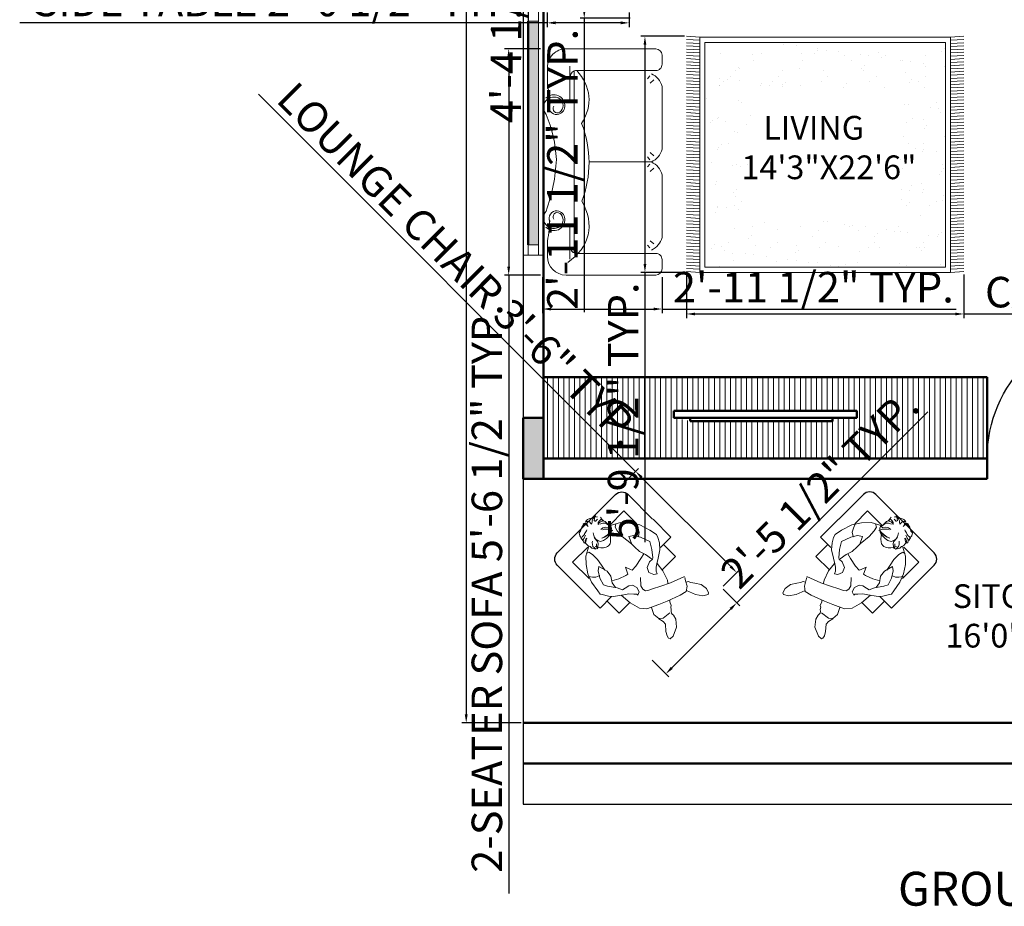
# Model space of a CAD drawing. Units: inches. Extents: x 3064 to 19385, y 846 to 15425.
# Tile 1 of 108: x 3072 to 3363, y 850 to 1112. Entities that reach past the tile are written whole.
import ezdxf

# ---------------------------------------------------------------- set-up
doc = ezdxf.new("R2010")
doc.units = ezdxf.units.IN
for name, color, linetype, lineweight in [('A-ANNO-DIMS', 2, 'Continuous', 18), ('A-ANNO-TEXT', 7, 'Continuous', 25), ('A-AREA-IDEN', 3, 'Continuous', 18), ('A-COLS', 1, 'Continuous', 35), ('A-DOOR', 3, 'Continuous', 25), ('A-FURN', 8, 'Continuous', 18), ('A-FURN-PATT', 252, 'Continuous', 13), ('A-GLAZ', 4, 'Continuous', 18), ('A-WALL', 7, 'Continuous', 50), ('C-PROP', 6, 'Continuous', 25)]:
    doc.layers.add(name, color=color, linetype=linetype, lineweight=lineweight)
doc.layers.add('NOITHAT', color=21, linetype='Continuous')
doc.styles.get("Standard").update_dxf_attribs({"font": 'arial.ttf'})
doc.dimstyles.new('ISO-25', dxfattribs={"dimtxt": 9, "dimasz": 2.5, "dimexe": 1.25, "dimexo": 0.625, "dimtad": 1, "dimdec": 1, "dimlunit": 3, "dimtxsty": 'Standard', "dimcen": 2.5, "dimadec": 0, "dimazin": 0, "dimtfac": 1, "dimtdec": 1, "dimtmove": 0, "dimatfit": 3, "dimfxl": 1, "dimarcsym": 0})

# ---------------------------------------------------------------- blocks, each defined once
blk = doc.blocks.new('*U2')
for p, q in [((0, 0), (0, -6)), ((40, 0), (40, -6))]:
    blk.add_line(p, q)
blk.add_lwpolyline([(0, 0), (0, 40), (1.75, 40), (1.75, 0)], close=True)
blk.add_arc((0, 0), 40, 0, 90)
blk = doc.blocks.new('carpet-9')
at = {"color": 0, "linetype": 'ByBlock'}
for p, q in [((-2.523, -0.142), (-2.531, 0)), ((-2.488, -0.142), (-2.497, 0)), ((-2.454, -0.142), (-2.462, 0)), ((-2.42, -0.142), (-2.428, 0)), ((-2.386, -0.142), (-2.394, 0)), ((-2.352, -0.142), (-2.36, 0)), ((-2.317, -0.142), (-2.326, 0)), ((-2.283, -0.142), (-2.291, 0)), ((-2.249, -0.142), (-2.257, 0)), ((-2.215, -0.142), (-2.223, 0)), ((-2.181, -0.142), (-2.189, 0)), ((-2.146, -0.142), (-2.155, 0)), ((-2.112, -0.142), (-2.12, 0)), ((-2.078, -0.142), (-2.086, 0)), ((-2.044, -0.142), (-2.052, 0)), ((-2.01, -0.142), (-2.018, 0)), ((-1.975, -0.142), (-1.984, 0)), ((-1.941, -0.142), (-1.949, 0)), ((-1.907, -0.142), (-1.915, 0)), ((-1.873, -0.142), (-1.881, 0)), ((-1.839, -0.142), (-1.847, 0)), ((-1.804, -0.142), (-1.813, 0)), ((-1.77, -0.142), (-1.778, 0)), ((-1.736, -0.142), (-1.744, 0)), ((-1.702, -0.142), (-1.71, 0)), ((-1.668, -0.142), (-1.676, 0)), ((-1.633, -0.142), (-1.642, 0)), ((-1.599, -0.142), (-1.607, 0)), ((-1.565, -0.142), (-1.573, 0)), ((-1.531, -0.142), (-1.539, 0)), ((-1.497, -0.142), (-1.505, 0)), ((-1.462, -0.142), (-1.471, 0)), ((-1.428, -0.142), (-1.436, 0)), ((-1.394, -0.142), (-1.402, 0)), ((-1.36, -0.142), (-1.368, 0)), ((-1.326, -0.142), (-1.334, 0)), ((-1.291, -0.142), (-1.3, 0)), ((-1.257, -0.142), (-1.265, 0)), ((-1.223, -0.142), (-1.231, 0)), ((-1.189, -0.142), (-1.197, 0)), ((-1.155, -0.142), (-1.163, 0)), ((-1.12, -0.142), (-1.129, 0)), ((-1.086, -0.142), (-1.094, 0)), ((-1.052, -0.142), (-1.06, 0)), ((-1.018, -0.142), (-1.026, 0)), ((-0.984, -0.142), (-0.992, 0)), ((-0.949, -0.142), (-0.958, 0)), ((-0.915, -0.142), (-0.923, 0)), ((-0.881, -0.142), (-0.889, 0)), ((-0.847, -0.142), (-0.855, 0)), ((-0.813, -0.142), (-0.821, 0)), ((-0.778, -0.142), (-0.787, 0)), ((-0.744, -0.142), (-0.752, 0)), ((-0.71, -0.142), (-0.718, 0)), ((-0.676, -0.142), (-0.684, 0)), ((-0.642, -0.142), (-0.65, 0)), ((-0.607, -0.142), (-0.616, 0)), ((-0.573, -0.142), (-0.581, 0)), ((-0.539, -0.142), (-0.547, 0)), ((-0.505, -0.142), (-0.513, 0)), ((-0.471, -0.142), (-0.479, 0)), ((-0.436, -0.142), (-0.445, 0)), ((-0.402, -0.142), (-0.41, 0)), ((-0.368, -0.142), (-0.376, 0)), ((-0.334, -0.142), (-0.342, 0)), ((-0.3, -0.142), (-0.308, 0)), ((-0.265, -0.142), (-0.274, 0)), ((-0.231, -0.142), (-0.239, 0)), ((-0.197, -0.142), (-0.205, 0)), ((-0.163, -0.142), (-0.171, 0)), ((-0.129, -0.142), (-0.137, 0)), ((-0.094, -0.142), (-0.103, 0)), ((-0.06, -0.142), (-0.068, 0)), ((-0.026, -0.142), (-0.034, 0)), ((0.008, -0.142), (0, 0)), ((0.008, -0.142), (-2.523, -0.142)), ((-2.523, -0.142), (-2.523, -2.842)), ((-0.049, -0.196), (-2.466, -0.196)), ((-2.466, -0.196), (-2.466, -2.788)), ((-2.206, -0.208), (-2.206, -0.208)), ((-1.451, -0.207), (-1.451, -0.207)), ((-0.049, -2.788), (-0.049, -0.196)), ((0.008, -2.842), (0.008, -0.142)), ((-2.396, -0.212), (-2.396, -0.212)), ((-2.365, -0.244), (-2.365, -0.244)), ((-1.82, -0.293), (-1.82, -0.293)), ((-1.754, -0.276), (-1.754, -0.276)), ((-1.712, -0.25), (-1.712, -0.25)), ((-1.296, -0.294), (-1.296, -0.294)), ((-1.153, -0.231), (-1.153, -0.231)), ((-1.108, -0.217), (-1.108, -0.217)), ((-1.079, -0.235), (-1.079, -0.235)), ((-1.049, -0.267), (-1.049, -0.267)), ((-0.824, -0.22), (-0.824, -0.22)), ((-0.765, -0.228), (-0.765, -0.228)), ((-0.755, -0.296), (-0.755, -0.296)), ((-0.421, -0.239), (-0.421, -0.239)), ((-0.396, -0.273), (-0.396, -0.273)), ((-0.373, -0.288), (-0.373, -0.288)), ((-0.078, -0.249), (-0.078, -0.249)), ((-2.322, -0.413), (-2.322, -0.413)), ((-2.203, -0.411), (-2.203, -0.411)), ((-2.094, -0.413), (-2.094, -0.413)), ((-1.979, -0.424), (-1.979, -0.424)), ((-1.767, -0.363), (-1.767, -0.363)), ((-1.57, -0.397), (-1.57, -0.397)), ((-0.707, -0.367), (-0.707, -0.367)), ((-0.385, -0.376), (-0.385, -0.376)), ((-0.254, -0.42), (-0.254, -0.42)), ((-2.238, -0.437), (-2.238, -0.437)), ((-2.046, -0.484), (-2.046, -0.484)), ((-1.635, -0.434), (-1.635, -0.434)), ((-1.54, -0.428), (-1.54, -0.428)), ((-1.374, -0.429), (-1.374, -0.429)), ((-1.327, -0.519), (-1.327, -0.519)), ((-1.315, -0.431), (-1.315, -0.431)), ((-1.292, -0.445), (-1.292, -0.445)), ((-0.949, -0.456), (-0.949, -0.456)), ((-0.887, -0.435), (-0.887, -0.435)), ((-0.856, -0.45), (-0.856, -0.45)), ((-0.606, -0.466), (-0.606, -0.466)), ((-0.309, -0.433), (-0.309, -0.433)), ((-0.263, -0.477), (-0.263, -0.477)), ((-0.261, -0.504), (-0.261, -0.504)), ((-0.224, -0.451), (-0.224, -0.451)), ((-2.257, -0.574), (-2.257, -0.574)), ((-2.144, -0.627), (-2.144, -0.627)), ((-2.061, -0.558), (-2.061, -0.558)), ((-2.031, -0.589), (-2.031, -0.589)), ((-1.799, -0.593), (-1.799, -0.593)), ((-1.648, -0.549), (-1.648, -0.549)), ((-1.6, -0.62), (-1.6, -0.62)), ((-1.378, -0.596), (-1.378, -0.596)), ((-0.928, -0.566), (-0.928, -0.566)), ((-0.875, -0.587), (-0.875, -0.587)), ((-0.745, -0.581), (-0.745, -0.581)), ((-0.715, -0.612), (-0.715, -0.612)), ((-0.417, -0.605), (-0.417, -0.605)), ((-0.061, -0.619), (-0.061, -0.619)), ((-2.269, -0.662), (-2.269, -0.662)), ((-2.268, -0.682), (-2.268, -0.682)), ((-1.8, -0.638), (-1.8, -0.638)), ((-1.457, -0.649), (-1.457, -0.649)), ((-1.202, -0.686), (-1.202, -0.686)), ((-1.114, -0.659), (-1.114, -0.659)), ((-0.888, -0.675), (-0.888, -0.675)), ((-0.771, -0.67), (-0.771, -0.67)), ((-0.482, -0.702), (-0.482, -0.702)), ((-0.427, -0.68), (-0.427, -0.68)), ((-0.084, -0.691), (-0.084, -0.691)), ((-2.32, -0.845), (-2.32, -0.845)), ((-0.448, -0.83), (-0.448, -0.83)), ((-0.436, -0.742), (-0.436, -0.742)), ((-2.359, -0.919), (-2.359, -0.919)), ((-2.301, -0.891), (-2.301, -0.891)), ((-2.095, -0.938), (-2.095, -0.938)), ((-1.976, -0.855), (-1.976, -0.855)), ((-0.41, -0.927), (-0.41, -0.927)), ((-0.26, -0.909), (-0.26, -0.909)), ((-2.32, -1.028), (-2.32, -1.028)), ((-2.047, -1.01), (-2.047, -1.01)), ((-0.48, -1.059), (-0.48, -1.059)), ((-0.38, -0.958), (-0.38, -0.958)), ((-0.31, -0.958), (-0.31, -0.958)), ((-0.262, -1.029), (-0.262, -1.029)), ((-2.332, -1.116), (-2.332, -1.116)), ((-2.217, -1.066), (-2.217, -1.066)), ((-2.187, -1.097), (-2.187, -1.097)), ((-2.161, -1.083), (-2.161, -1.083)), ((-0.445, -1.136), (-0.445, -1.136)), ((-0.218, -1.126), (-0.218, -1.126)), ((-0.102, -1.147), (-0.102, -1.147)), ((-2.269, -1.208), (-2.269, -1.208)), ((-2.025, -1.265), (-2.025, -1.265)), ((-0.499, -1.197), (-0.499, -1.197)), ((-0.483, -1.227), (-0.483, -1.227)), ((-2.364, -1.346), (-2.364, -1.346)), ((-2.326, -1.287), (-2.326, -1.287)), ((-1.982, -1.297), (-1.982, -1.297)), ((-0.511, -1.284), (-0.511, -1.284)), ((-0.266, -1.35), (-0.266, -1.35)), ((-0.076, -1.273), (-0.076, -1.273)), ((-0.059, -1.352), (-0.059, -1.352)), ((-2.383, -1.483), (-2.383, -1.483)), ((-2.096, -1.464), (-2.096, -1.464)), ((-0.536, -1.466), (-0.536, -1.466)), ((-0.311, -1.484), (-0.311, -1.484)), ((-0.071, -1.44), (-0.071, -1.44)), ((-2.396, -1.571), (-2.396, -1.571)), ((-2.374, -1.573), (-2.374, -1.573)), ((-2.159, -1.515), (-2.159, -1.515)), ((-2.048, -1.535), (-2.048, -1.535)), ((-0.543, -1.514), (-0.543, -1.514)), ((-0.443, -1.568), (-0.443, -1.568)), ((-0.263, -1.555), (-0.263, -1.555)), ((-0.099, -1.579), (-0.099, -1.579)), ((-2.344, -1.604), (-2.344, -1.604)), ((-0.374, -1.634), (-0.374, -1.634)), ((-0.103, -1.669), (-0.103, -1.669)), ((-2.427, -1.8), (-2.427, -1.8)), ((-2.343, -1.742), (-2.343, -1.742)), ((-2.27, -1.733), (-2.27, -1.733)), ((-2.181, -1.772), (-2.181, -1.772)), ((-2, -1.753), (-2, -1.753)), ((-0.484, -1.753), (-0.484, -1.753)), ((-0.232, -1.78), (-0.232, -1.78)), ((-0.284, -1.806), (-0.284, -1.806)), ((-0.202, -1.811), (-0.202, -1.811)), ((-0.135, -1.894), (-0.135, -1.894)), ((-0.122, -1.806), (-0.122, -1.806)), ((-2.447, -1.937), (-2.447, -1.937)), ((-2.165, -1.956), (-2.165, -1.956)), ((-2.097, -1.99), (-2.097, -1.99)), ((-2.039, -1.919), (-2.039, -1.919)), ((-2.009, -1.95), (-2.009, -1.95)), ((-1.988, -1.955), (-1.988, -1.955)), ((-0.449, -2.01), (-0.449, -2.01)), ((-0.312, -2.009), (-0.312, -2.009)), ((-2.459, -2.025), (-2.459, -2.025)), ((-2.049, -2.061), (-2.049, -2.061)), ((-2.007, -2.093), (-2.007, -2.093)), ((-0.264, -2.08), (-0.264, -2.08)), ((-0.105, -2.02), (-0.105, -2.02)), ((-2.341, -2.174), (-2.341, -2.174)), ((-2.019, -2.18), (-2.019, -2.18)), ((-1.998, -2.185), (-1.998, -2.185)), ((-0.53, -2.141), (-0.53, -2.141)), ((-0.166, -2.123), (-0.166, -2.123)), ((-2.337, -2.279), (-2.337, -2.279)), ((-2.271, -2.259), (-2.271, -2.259)), ((-1.674, -2.296), (-1.674, -2.296)), ((-1.021, -2.302), (-1.021, -2.302)), ((-0.485, -2.278), (-0.485, -2.278)), ((-0.388, -2.288), (-0.388, -2.288)), ((-0.358, -2.319), (-0.358, -2.319)), ((-0.282, -2.238), (-0.282, -2.238)), ((-0.186, -2.261), (-0.186, -2.261)), ((-2.195, -2.426), (-2.195, -2.426)), ((-2.182, -2.412), (-2.182, -2.412)), ((-2.051, -2.41), (-2.051, -2.41)), ((-1.839, -2.423), (-1.839, -2.423)), ((-1.824, -2.395), (-1.824, -2.395)), ((-1.58, -2.336), (-1.58, -2.336)), ((-1.496, -2.434), (-1.496, -2.434)), ((-1.157, -2.333), (-1.157, -2.333)), ((-1.128, -2.404), (-1.128, -2.404)), ((-0.759, -2.398), (-0.759, -2.398)), ((-0.669, -2.422), (-0.669, -2.422)), ((-0.198, -2.348), (-0.198, -2.348)), ((-2.165, -2.457), (-2.165, -2.457)), ((-2.098, -2.515), (-2.098, -2.515)), ((-1.512, -2.464), (-1.512, -2.464)), ((-1.378, -2.531), (-1.378, -2.531)), ((-1.152, -2.444), (-1.152, -2.444)), ((-1.14, -2.492), (-1.14, -2.492)), ((-0.879, -2.449), (-0.879, -2.449)), ((-0.849, -2.48), (-0.849, -2.48)), ((-0.809, -2.455), (-0.809, -2.455)), ((-0.711, -2.47), (-0.711, -2.47)), ((-0.466, -2.465), (-0.466, -2.465)), ((-0.313, -2.535), (-0.313, -2.535)), ((-0.196, -2.487), (-0.196, -2.487)), ((-0.123, -2.476), (-0.123, -2.476)), ((-2.347, -2.616), (-2.347, -2.616)), ((-2.082, -2.635), (-2.082, -2.635)), ((-2.07, -2.547), (-2.07, -2.547)), ((-2.05, -2.586), (-2.05, -2.586)), ((-2.004, -2.626), (-2.004, -2.626)), ((-2.003, -2.625), (-2.003, -2.625)), ((-1.66, -2.637), (-1.66, -2.637)), ((-1.611, -2.565), (-1.611, -2.565)), ((-1.37, -2.61), (-1.37, -2.61)), ((-1.34, -2.642), (-1.34, -2.642)), ((-1.317, -2.648), (-1.317, -2.648)), ((-0.7, -2.647), (-0.7, -2.647)), ((-0.688, -2.559), (-0.688, -2.559)), ((-0.687, -2.648), (-0.687, -2.648)), ((-0.265, -2.606), (-0.265, -2.606)), ((-0.23, -2.578), (-0.23, -2.578)), ((-0.054, -2.634), (-0.054, -2.634)), ((-1.652, -2.651), (-1.652, -2.651)), ((-1.63, -2.702), (-1.63, -2.702)), ((-1.604, -2.722), (-1.604, -2.722)), ((-1.172, -2.721), (-1.172, -2.721)), ((-0.974, -2.658), (-0.974, -2.658)), ((-0.932, -2.668), (-0.932, -2.668)), ((-0.631, -2.669), (-0.631, -2.669)), ((-0.287, -2.68), (-0.287, -2.68)), ((-0.249, -2.715), (-0.249, -2.715)), ((-2.523, -2.842), (-2.531, -2.985)), ((-2.523, -2.842), (0.008, -2.842)), ((-2.488, -2.842), (-2.497, -2.985)), ((-2.466, -2.788), (-0.049, -2.788)), ((-2.454, -2.842), (-2.462, -2.985)), ((-2.42, -2.842), (-2.428, -2.985)), ((-2.386, -2.842), (-2.394, -2.985)), ((-2.352, -2.842), (-2.36, -2.985)), ((-2.317, -2.842), (-2.326, -2.985)), ((-2.283, -2.842), (-2.291, -2.985)), ((-2.272, -2.784), (-2.272, -2.784)), ((-2.249, -2.842), (-2.257, -2.985)), ((-2.215, -2.842), (-2.223, -2.985)), ((-2.181, -2.842), (-2.189, -2.985)), ((-2.146, -2.842), (-2.155, -2.985)), ((-2.112, -2.842), (-2.12, -2.985)), ((-2.078, -2.842), (-2.086, -2.985)), ((-2.044, -2.842), (-2.052, -2.985)), ((-2.01, -2.842), (-2.018, -2.985)), ((-1.975, -2.842), (-1.984, -2.985)), ((-1.941, -2.842), (-1.949, -2.985)), ((-1.907, -2.842), (-1.915, -2.985)), ((-1.873, -2.842), (-1.881, -2.985)), ((-1.861, -2.772), (-1.861, -2.772)), ((-1.839, -2.842), (-1.847, -2.985)), ((-1.804, -2.842), (-1.813, -2.985)), ((-1.77, -2.842), (-1.778, -2.985)), ((-1.736, -2.842), (-1.744, -2.985)), ((-1.702, -2.842), (-1.71, -2.985)), ((-1.668, -2.842), (-1.676, -2.985)), ((-1.633, -2.842), (-1.642, -2.985)), ((-1.599, -2.842), (-1.607, -2.985)), ((-1.565, -2.842), (-1.573, -2.985)), ((-1.531, -2.842), (-1.539, -2.985)), ((-1.497, -2.842), (-1.505, -2.985)), ((-1.462, -2.842), (-1.471, -2.985)), ((-1.428, -2.842), (-1.436, -2.985)), ((-1.394, -2.842), (-1.402, -2.985)), ((-1.36, -2.842), (-1.368, -2.985)), ((-1.326, -2.842), (-1.334, -2.985)), ((-1.291, -2.842), (-1.3, -2.985)), ((-1.257, -2.842), (-1.265, -2.985)), ((-1.223, -2.842), (-1.231, -2.985)), ((-1.206, -2.788), (-1.206, -2.788)), ((-1.189, -2.842), (-1.197, -2.985)), ((-1.155, -2.842), (-1.163, -2.985)), ((-1.12, -2.842), (-1.129, -2.985)), ((-1.086, -2.842), (-1.094, -2.985)), ((-1.052, -2.842), (-1.06, -2.985)), ((-1.018, -2.842), (-1.026, -2.985)), ((-0.984, -2.842), (-0.992, -2.985)), ((-0.949, -2.842), (-0.958, -2.985)), ((-0.915, -2.842), (-0.923, -2.985)), ((-0.881, -2.842), (-0.889, -2.985)), ((-0.847, -2.842), (-0.855, -2.985)), ((-0.813, -2.842), (-0.821, -2.985)), ((-0.778, -2.842), (-0.787, -2.985)), ((-0.744, -2.842), (-0.752, -2.985)), ((-0.71, -2.842), (-0.718, -2.985)), ((-0.676, -2.842), (-0.684, -2.985)), ((-0.642, -2.842), (-0.65, -2.985)), ((-0.607, -2.842), (-0.616, -2.985)), ((-0.573, -2.842), (-0.581, -2.985)), ((-0.539, -2.842), (-0.547, -2.985)), ((-0.505, -2.842), (-0.513, -2.985)), ((-0.471, -2.842), (-0.479, -2.985)), ((-0.436, -2.842), (-0.445, -2.985)), ((-0.402, -2.842), (-0.41, -2.985)), ((-0.368, -2.842), (-0.376, -2.985)), ((-0.334, -2.842), (-0.342, -2.985)), ((-0.3, -2.842), (-0.308, -2.985)), ((-0.265, -2.842), (-0.274, -2.985)), ((-0.231, -2.842), (-0.239, -2.985)), ((-0.197, -2.842), (-0.205, -2.985)), ((-0.163, -2.842), (-0.171, -2.985)), ((-0.129, -2.842), (-0.137, -2.985)), ((-0.094, -2.842), (-0.103, -2.985)), ((-0.06, -2.842), (-0.068, -2.985)), ((-0.026, -2.842), (-0.034, -2.985)), ((0.008, -2.842), (0, -2.985))]:
    blk.add_line(p, q, dxfattribs=at)
blk = doc.blocks.new('sofa-33')
at = {"color": 0, "linetype": 'ByBlock'}
for p, q in [((-0.15, 0.15), (-0.15, 0.8738)), ((-0.026, 0.9238), (-0.1, 0.9238)), ((0.024, 0.2361), (0.024, 0.8738)), ((0.657, 0.9252), (0.1531, 0.9252)), ((0.8633, 0.9252), (1.3671, 0.9252)), ((1.4963, 0.2361), (1.4963, 0.8738)), ((1.6203, 0.9238), (1.5463, 0.9238)), ((1.6703, 0.15), (1.6703, 0.8738)), ((0.05, 0.8375), (0.05, 0.8379)), ((0.0903, 0.8062), (0.0682, 0.8242)), ((0.1006, 0.8574), (0.1265, 0.8286)), ((0.7096, 0.8574), (0.6837, 0.8286)), ((0.7199, 0.8062), (0.742, 0.8242)), ((0.7602, 0.8375), (0.7601, 0.8379)), ((0.7601, 0.8375), (0.7601, 0.8379)), ((0.7602, 0.8375), (0.7602, 0.3356)), ((0.8004, 0.8062), (0.7783, 0.8242)), ((0.8107, 0.8574), (0.8366, 0.8286)), ((1.4197, 0.8574), (1.3938, 0.8286)), ((1.43, 0.8062), (1.4521, 0.8242)), ((1.4702, 0.8375), (1.4703, 0.8379)), ((1.4702, 0.8375), (1.4703, 0.8379)), ((-0.01, 0.1801), (0.2738, 0.1801)), ((0.0289, 0.2145), (1.4914, 0.2145)), ((1.5422, 0.1801), (1.2585, 0.1801)), ((0, 0), (0.1356, 0)), ((1.5322, 0), (1.3966, 0))]:
    blk.add_line(p, q, dxfattribs=at)
at = {"color": 0, "linetype": 'ByBlock', "extrusion": (0, 0, -1)}
for centre, major_axis, ratio, start_param, end_param in [((-0.1, 0.8738), (0.0354, 0.0354), 1, 3.926992, 5.497787), ((-0.026, 0.8738), (-0.0354, 0.0354), 1, 0.785398, 2.356196), ((0.1997, 0.7661), (0.1173, 0.1173), 1, 4.372209, 5.213218), ((0.6105, 0.7661), (0.1173, 0.1173), 1, -0.500829, 0.34018), ((0.9098, 0.7661), (0.1173, 0.1173), 1, 4.372209, 5.213218), ((1.3206, 0.7661), (-0.1173, 0.1173), 1, 1.069968, 1.910976), ((1.5463, 0.8738), (-0.0354, 0.0354), 1, 5.497786, 7.068583), ((1.6203, 0.8738), (0.0354, 0.0354), 1, -0.785398, 0.785398), ((0.3234, -0.6657), (-0.0931, 0.9998), 0.551284, -0.397889, 0.397889), ((0.7664, -0.6685), (-0.0034, 1.0041), 0.922365, -0.343589, 0.343589), ((1.147, -0.5336), (0.1998, 0.8608), 0.59532, -0.502747, 0.502747), ((0.074, 0.2361), (-0.0354, 0.0354), 1, 3.926991, 5.497788), ((1.4463, 0.2361), (0.0354, 0.0354), 1, 0.785397, 2.356194), ((0, 0.15), (0.1061, 0.1061), 1, 2.356194, 3.926992), ((0.3076, 0.0525), (-0.0624, 0.0624), 1, 4.675944, 7.152385), ((0.3208, 0.0524), (-0.059, 0.059), 1, 3.186406, 6.094039), ((0.3052, 0.0629), (-0.0458, 0.0458), 1, 6.094039, 8.043134), ((0.3201, 0.0726), (-0.0414, 0.0414), 1, 2.230507, 4.423483), ((0.3301, 0.0798), (0.0245, 0.0245), 1, 0.189152, 2.952444), ((0.3092, 0.0712), (0.0491, 0.0491), 1, -0.701597, 0.659711), ((1.2122, 0.0726), (-0.0414, 0.0414), 1, 3.430501, 5.623477), ((1.223, 0.0712), (-0.0491, 0.0491), 1, 5.623477, 6.984784), ((1.2115, 0.0524), (0.059, 0.059), 1, 0.189149, 3.096782), ((1.2022, 0.0798), (0.0245, 0.0245), 1, 1.759947, 4.52324), ((1.227, 0.0629), (0.0458, 0.0458), 1, 4.52324, 6.472335), ((1.2246, 0.0525), (-0.0624, 0.0624), 1, 0.701599, 3.17804), ((1.5203, 0.15), (0.1061, 0.1061), 1, 0.785398, 2.356194), ((0.2824, -0.6613), (-0.479, 0.479), 1, 0.566947, 0.842011), ((0.8779, -1.3822), (-0.3228, 1.4289), 0.878591, -0.144977, 0.144977), ((0.6669, -1.3904), (1.0359, 1.0359), 1, 5.547613, 5.837566), ((1.2498, -0.6613), (0.479, 0.479), 1, 5.441177, 5.716241)]:
    blk.add_ellipse(centre, major_axis=major_axis, ratio=ratio, start_param=start_param, end_param=end_param, dxfattribs=at)
blk = doc.blocks.new('A$C48E80792')
for p, q in [((208.1, 777.4), (217.7, 791.8)), ((217.7, 791.8), (230.8, 792.5)), ((230.8, 792.5), (252, 804.1)), ((252, 804.1), (267.8, 807.6)), ((253.5, 801.9), (261.1, 805.7)), ((261.1, 805.7), (274.4, 805.7)), ((267.8, 807.6), (270.5, 811.7)), ((284, 805.7), (270.6, 811.4)), ((274.4, 805.7), (278.3, 805.7)), ((278.3, 805.7), (278.3, 798.1)), ((278.3, 798.1), (280.2, 788.5)), ((280.2, 786.6), (284, 794.3)), ((280.2, 788.5), (280.2, 780.9)), ((280.2, 780.9), (280.2, 786.6)), ((284, 794.3), (284, 805.7)), ((289.7, 811.4), (305.5, 811.7)), ((289.7, 811.4), (303, 796.2)), ((303, 796.2), (303, 779)), ((303, 777.1), (312.6, 782.8)), ((305.5, 811.7), (317.9, 805.5)), ((312.6, 782.8), (318.3, 788.5)), ((317.9, 805.5), (328.1, 800)), ((318.3, 788.5), (329.8, 792.4)), ((335.5, 786.6), (327.8, 780.9)), ((328.1, 800), (343.9, 798)), ((329.8, 792.4), (343.1, 794.3)), ((343.1, 792.4), (335.5, 786.6)), ((343.1, 794.3), (352.6, 794.3)), ((352.6, 792.4), (343.1, 792.4)), ((343.9, 798), (352.1, 795.9)), ((343.9, 790.4), (354.9, 782.2)), ((198.1, 735.2), (202, 742.8)), ((198.1, 727.5), (198.1, 735.2)), ((202, 727.5), (200.1, 725.6)), ((202, 746.6), (204.7, 764.4)), ((202, 746.6), (205.8, 759.9)), ((202, 742.8), (207.7, 748.5)), ((211.5, 737.1), (202, 727.5)), ((202, 723.7), (209.6, 729.4)), ((204.7, 764.4), (207.4, 769.9)), ((205.8, 759.9), (213.4, 763.8)), ((207.4, 769.9), (208.1, 777.4)), ((207.7, 748.5), (217.2, 750.4)), ((209.6, 729.4), (219.1, 735.2)), ((219.1, 739), (211.5, 737.1)), ((213.4, 763.8), (222.9, 763.8)), ((217.2, 750.4), (226.8, 754.2)), ((226.8, 739), (219.1, 739)), ((219.1, 735.2), (226.8, 739)), ((222.9, 763.8), (232.5, 763.8)), ((226.8, 754.2), (234.4, 756.1)), ((226.8, 739), (226.8, 739)), ((232.5, 763.8), (236.3, 765.7)), ((236.3, 765.7), (242, 767.6)), ((242, 767.6), (255.4, 771.4)), ((255.4, 771.4), (261.1, 773.3)), ((274, 735.6), (261.6, 715.7)), ((303, 779), (303, 777.1)), ((327.8, 780.9), (327.8, 775.2)), ((327.8, 748.5), (335.5, 756.1)), ((329.8, 748.5), (327.8, 748.5)), ((329.8, 771.4), (335.5, 773.3)), ((335.5, 750.4), (329.8, 748.5)), ((335.5, 773.3), (346.9, 773.3)), ((335.5, 756.1), (346.9, 758)), ((337.4, 750.4), (335.5, 750.4)), ((352.6, 735.2), (335.5, 742.8)), ((341.2, 750.4), (337.4, 750.4)), ((346.9, 750.4), (341.2, 750.4)), ((346.9, 758), (358.4, 758)), ((354.5, 746.6), (346.9, 750.4)), ((356.5, 731.3), (352.6, 735.2)), ((362.2, 742.8), (354.5, 746.6)), ((362.2, 750.4), (356.5, 746.6)), ((362.2, 723.7), (356.5, 731.3)), ((358.4, 758), (362.2, 756.1)), ((366, 769.5), (362.2, 750.4)), ((362.2, 756.1), (364.1, 750.4)), ((367.9, 733.3), (362.2, 742.8)), ((364.1, 750.4), (364.1, 742.8)), ((364.1, 742.8), (364.1, 739)), ((367.9, 706.6), (367.9, 733.3)), ((151.7, 671.2), (119.2, 637.1)), ((204, 699.4), (151.7, 671.2)), ((165.1, 679.5), (178.4, 675)), ((178.4, 675), (185.1, 650.5)), ((202, 716.1), (202, 723.7)), ((202, 706.6), (202, 716.1)), ((202, 702.8), (202, 706.6)), ((207.7, 693.2), (202, 702.8)), ((207.7, 679.9), (207.7, 693.2)), ((219.1, 658.9), (207.7, 679.9)), ((219.1, 681.8), (224.8, 691.3)), ((219.1, 670.3), (219.1, 681.8)), ((224.8, 691.3), (232.5, 700.8)), ((227.3, 673.2), (235.6, 655.4)), ((232.5, 700.8), (238.2, 704.7)), ((236.3, 670.3), (243.9, 678)), ((257.3, 679.9), (249.6, 670.3)), ((259.2, 708.5), (257.3, 679.9)), ((260.3, 708.9), (259.6, 699.3)), ((259.6, 699.3), (261.6, 685.6)), ((261.6, 715.7), (260.3, 708.9)), ((261.6, 685.6), (269.2, 671.8)), ((269.2, 671.8), (285.6, 662.9)), ((302.1, 672.5), (287, 679.4)), ((287, 679.4), (304.8, 673.9)), ((323.3, 667), (302.1, 672.5)), ((304.8, 673.9), (323.3, 670.5)), ((318.3, 718), (333.6, 716.1)), ((331.7, 706.6), (324, 710.4)), ((339.3, 700.8), (331.7, 706.6)), ((333.6, 716.1), (339.3, 712.3)), ((339.3, 712.3), (346.9, 708.5)), ((346.9, 693.2), (339.3, 700.8)), ((346.9, 708.5), (358.4, 695.1)), ((354.5, 685.6), (346.9, 693.2)), ((356.5, 676.1), (354.5, 685.6)), ((356.3, 668.4), (367.2, 680.1)), ((362.2, 666.5), (356.5, 676.1)), ((358.4, 695.1), (360.3, 693.2)), ((360.3, 693.2), (366, 691.3)), ((364.1, 718), (362.2, 723.7)), ((366, 706.6), (364.1, 718)), ((367.9, 698.9), (366, 706.6)), ((366, 691.3), (369.8, 689.4)), ((366.5, 698.9), (425.1, 668)), ((367.2, 680.1), (370.7, 689)), ((371.7, 691.3), (367.9, 698.9)), ((369.8, 689.4), (371.7, 689.4)), ((371.7, 689.4), (371.7, 691.3)), ((371.7, 689.4), (371.7, 689.4)), ((401.2, 679.5), (385.6, 670.5)), ((119.2, 637.1), (88.2, 591.5)), ((185.1, 650.5), (185.1, 610.4)), ((221, 657), (219.1, 670.3)), ((226.8, 655.1), (232.5, 664.6)), ((232.5, 657), (226.8, 655.1)), ((232.5, 664.6), (236.3, 670.3)), ((238.2, 660.8), (232.5, 657)), ((235.6, 655.4), (243.8, 644.4)), ((249.6, 670.3), (238.2, 660.8)), ((243.8, 644.4), (254.8, 633.5)), ((254.8, 633.5), (267.8, 625.9)), ((267.8, 625.9), (276.7, 622.5)), ((276.7, 622.5), (283.6, 621.8)), ((283.6, 621.8), (298, 623.9)), ((285.6, 662.9), (304.8, 659.5)), ((298, 623.9), (307.6, 630.7)), ((304.8, 659.5), (326.8, 659.5)), ((307.6, 630.7), (319.2, 640.3)), ((319.2, 640.3), (330.9, 654)), ((323.3, 670.5), (345.3, 668.4)), ((337.7, 666.4), (323.3, 667)), ((326.8, 659.5), (340.5, 661.6)), ((330.9, 654), (334, 660.6)), ((356.3, 669.8), (337.7, 666.4)), ((340.5, 661.6), (348.7, 664.3)), ((345.3, 668.4), (356.3, 668.4)), ((348.7, 664.3), (352.1, 667.7)), ((352.1, 667.7), (356.3, 669.8)), ((356.3, 668.4), (358.3, 669.8)), ((378.9, 646.1), (376.7, 603.8)), ((385.6, 670.5), (378.9, 646.1)), ((425.1, 668), (462.5, 627.3)), ((462.5, 627.3), (493.4, 580.1)), ((88.2, 591.5), (70.3, 544.3)), ((80.4, 579.3), (93.8, 559.2)), ((93.8, 559.2), (107.1, 545.9)), ((119.2, 526.5), (141.9, 562.2)), ((141.9, 562.2), (161.5, 576.9)), ((161.5, 576.9), (175.7, 525.7)), ((178.4, 572.6), (171.7, 539.2)), ((185.1, 610.4), (178.4, 572.6)), ((376.7, 603.8), (383.3, 537)), ((402.3, 576.9), (383.3, 535)), ((426.7, 560.6), (402.3, 576.9)), ((447.9, 528.1), (426.7, 560.6)), ((472.4, 574.8), (461.3, 552.6)), ((485.8, 606), (472.4, 574.8)), ((493.4, 580.1), (513, 518.3)), ((70.3, 544.3), (60.6, 484.2)), ((106.8, 485.6), (119.2, 526.5)), ((107.1, 545.9), (125, 539.2)), ((125, 539.2), (129.4, 537)), ((175.7, 525.7), (172, 490.5)), ((383.3, 535), (383.3, 512.7)), ((383.3, 512.7), (385.2, 475.7)), ((461.3, 552.6), (441.3, 539.2)), ((441.3, 539.2), (441.3, 537)), ((467.4, 472.8), (447.9, 528.1)), ((513, 518.3), (521.1, 474.4)), ((60.6, 484.2), (55.7, 461.4)), ((55.7, 461.4), (62.2, 451.6)), ((62.2, 451.6), (81.7, 419.1)), ((117.5, 463), (106.8, 485.6)), ((149.1, 418.9), (117.5, 463)), ((149.7, 459), (143.7, 426.5)), ((172, 490.5), (149.7, 459)), ((156.1, 468), (191.8, 447.9)), ((191.8, 447.9), (234.1, 432.3)), ((247.5, 430.1), (265.3, 468)), ((265.3, 468), (276.4, 439)), ((363.3, 441.2), (392.3, 447.9)), ((385.2, 475.7), (396.3, 438.6)), ((443, 432.1), (467.4, 472.8)), ((514.6, 456.5), (499.9, 428.9)), ((521.1, 474.4), (514.6, 456.5)), ((81.7, 419.1), (99.6, 398)), ((99.6, 398), (147.5, 363.6)), ((163.7, 389.7), (149.1, 418.9)), ((234.1, 432.3), (247.5, 430.1)), ((276.4, 439), (280.9, 427.9)), ((280.9, 427.9), (312.1, 430.1)), ((312.1, 430.1), (363.3, 441.2)), ((351.9, 380.1), (382.8, 393.1)), ((382.8, 393.1), (405.6, 391.5)), ((396.3, 438.6), (403.7, 397.8)), ((405.6, 391.5), (413.7, 396.3)), ((413.7, 396.3), (443, 432.1)), ((473.9, 399.6), (433.2, 373.6)), ((499.9, 428.9), (473.9, 399.6)), ((136.8, 373.8), (142.3, 307)), ((147.5, 363.6), (171.9, 347.4)), ((180, 384.8), (163.7, 389.7)), ((171.9, 347.4), (191.4, 326.2)), ((204.4, 379.9), (180, 384.8)), ((222.3, 368.5), (204.4, 379.9)), ((230.5, 340.9), (222.3, 368.5)), ((222.3, 313.2), (230.5, 340.9)), ((285.1, 367.1), (252.6, 331.3)), ((338.8, 352.4), (351.9, 380.1)), ((350.2, 324.8), (338.8, 352.4)), ((389.3, 345.9), (373, 329.7)), ((405.6, 355.7), (389.3, 345.9)), ((407.4, 355.2), (401.9, 303.3)), ((433.2, 373.6), (405.6, 355.7)), ((142.3, 307), (157.1, 247.7)), ((191.4, 326.2), (202.8, 314.8)), ((202.8, 314.8), (202.8, 306.7)), ((202.8, 306.7), (222.3, 313.2)), ((252.6, 331.3), (247.7, 310.1)), ((247.7, 310.1), (251, 292.3)), ((251, 292.3), (262.4, 284.1)), ((262.4, 284.1), (288.4, 272.7)), ((366.5, 315), (350.2, 324.8)), ((373, 329.7), (366.5, 315)), ((401.9, 303.3), (383.3, 247.7)), ((157.1, 247.7), (185, 214.4)), ((288.4, 272.7), (332.3, 250)), ((332.3, 250), (384.4, 223.9)), ((383.3, 247.7), (372.2, 232.9)), ((384.4, 223.9), (466, 193.4)), ((185, 214.4), (249.8, 184.7)), ((209.1, 201.4), (190.5, 164.4)), ((249.8, 184.7), (296.2, 164.4)), ((437.1, 144), (452.7, 171.9)), ((452.7, 171.9), (462.5, 188.2)), ((190.5, 164.4), (194.2, 129.2)), ((192.4, 126.7), (199, 98.4)), ((194.2, 129.2), (212.8, 112.5)), ((212.8, 112.5), (261.8, 106.9)), ((270.8, 106.7), (280.8, 115.1)), ((280.8, 115.1), (287.5, 125.1)), ((287.5, 125.1), (295.8, 130.1)), ((295.8, 130.1), (305.5, 151.4)), ((296.2, 164.4), (374.1, 136.6)), ((305.5, 151.4), (311, 157)), ((374.1, 136.6), (413, 127.3)), ((413, 127.3), (437.1, 144)), ((417.2, 129.7), (436.8, 77.9)), ((461.2, 158.8), (450.1, 164.4)), ((468.1, 144.2), (461.2, 158.8)), ((480.4, 126.2), (468.1, 144.2)), ((500.2, 94.8), (480.4, 126.2)), ((197.4, 78.4), (170.7, 48.4)), ((199, 98.4), (197.4, 78.4)), ((230.7, 21.7), (259.1, 56.7)), ((259.1, 56.7), (265.8, 83.4)), ((265.8, 98.4), (270.8, 106.7)), ((265.8, 91.7), (265.8, 98.4)), ((265.8, 83.4), (265.8, 91.7)), ((436.8, 77.9), (461.5, 41.9)), ((496.7, 31.6), (505.1, 56.7)), ((505.1, 56.7), (500.2, 94.8)), ((157.3, 25), (154, 10)), ((154, 10), (157.3, 1.7)), ((170.7, 48.4), (157.3, 25)), ((157.3, 1.7), (180.7, 0)), ((180.7, 0), (230.7, 21.7)), ((461.5, 41.9), (488.5, 26.9)), ((488.5, 26.9), (496.7, 31.6))]:
    blk.add_line(p, q)
blk.add_arc((337.3, 639.4), 150, 89.3152, 90)
at = {"layer": 'NOITHAT'}
for p, q in [((0.2, 550.4), (0, 405.9)), ((569, 405.9), (569.1, 549.9))]:
    blk.add_line(p, q, dxfattribs=at)
blk.add_lwpolyline([(0.1, 548.9), (0.1, 748.9, -0.414214), (50.1, 798.9), (518.1, 798.9, -0.414214), (568.1, 748.9), (568.1, 551.9)], format="xyb", dxfattribs=at)
for points in [[(195.1, 699.9), (74.1, 699.9), (74.1, 567.9)], [(486.1, 596.9), (486.1, 699.9), (369.1, 699.9)], [(92.1, 405.9), (0, 405.9)], [(56.1, 405.9), (56.1, 309.9), (142.1, 309.9)], [(402.6, 309.9), (510.1, 309.9), (510.1, 405.9)], [(486.1, 405.9), (569, 405.9)]]:
    blk.add_lwpolyline(points, dxfattribs=at)
blk = doc.blocks.new('*D39')
at = {"layer": 'A-ANNO-DIMS', "color": 0, "lineweight": -2, "transparency": 16777216}
for p, q in [((3220.22, 1396.34), (3202.78, 1396.34)), ((3204.03, 1393.84), (3204.03, 906.84)), ((3220.22, 904.34), (3202.78, 904.34))]:
    blk.add_line(p, q, dxfattribs=at)
at = {"layer": 'A-ANNO-DIMS', "color": 0, "transparency": 16777216}
for points in [[(3203.61, 1393.84), (3204.45, 1393.84), (3204.03, 1396.34)], [(3203.61, 906.84), (3204.45, 906.84), (3204.03, 904.34)]]:
    blk.add_solid(points, dxfattribs=at)
at = {"layer": 'Defpoints', "color": 0, "transparency": 16777216}
for p in [(3220.85, 1396.34), (3204.03, 904.34), (3220.85, 904.34)]:
    blk.add_point(p, dxfattribs=at)
at = {"layer": 'A-ANNO-DIMS', "color": 0, "transparency": 16777216, "insert": (3198.89, 1150.34), "char_height": 9, "attachment_point": 5, "rotation": 90}
blk.add_mtext("41'", dxfattribs=at)
blk = doc.blocks.new('WIN-1900')
blk.add_line((3, 0), (3, 66))
blk.add_lwpolyline([(3, 66), (0, 66), (0, 69), (3, 69)], close=True)
blk = doc.blocks.new('*D411')
at = {"layer": 'A-ANNO-DIMS', "color": 0, "lineweight": -2, "transparency": 16777216}
for p, q in [((3254.03, 978.55), (3142.72, 1089.86)), ((3249.99, 974.52), (3254.91, 979.44)), ((3282.12, 950.46), (3255.8, 976.78)), ((3279.85, 944.66), (3284.77, 949.58))]:
    blk.add_line(p, q, dxfattribs=at)
at = {"layer": 'A-ANNO-DIMS', "color": 0, "transparency": 16777216}
for points in [[(3256.09, 977.08), (3255.5, 976.49), (3254.03, 978.55)], [(3282.41, 950.76), (3281.82, 950.17), (3283.89, 948.7)]]:
    blk.add_solid(points, dxfattribs=at)
at = {"layer": 'Defpoints', "color": 0, "transparency": 16777216}
for p in [(3254.03, 978.55), (3249.55, 974.07), (3279.41, 944.22)]:
    blk.add_point(p, dxfattribs=at)
at = {"layer": 'A-ANNO-DIMS', "color": 0, "transparency": 16777216, "insert": (3201.23, 1038.83), "char_height": 9, "attachment_point": 5, "rotation": 315}
blk.add_mtext('LOUNGE CHAIR 3\'-6" TYP.', dxfattribs=at)
blk = doc.blocks.new('*D412')
at = {"layer": 'A-ANNO-DIMS', "color": 0, "lineweight": -2, "transparency": 16777216}
for p, q in [((3283.89, 939.74), (3340.27, 996.12)), ((3279.85, 943.78), (3284.77, 938.85)), ((3264.72, 920.57), (3282.12, 937.97)), ((3258.92, 922.84), (3263.84, 917.92))]:
    blk.add_line(p, q, dxfattribs=at)
at = {"layer": 'A-ANNO-DIMS', "color": 0, "transparency": 16777216}
for points in [[(3281.82, 938.27), (3282.41, 937.68), (3283.89, 939.74)], [(3264.42, 920.87), (3265.01, 920.28), (3262.95, 918.8)]]:
    blk.add_solid(points, dxfattribs=at)
at = {"layer": 'Defpoints', "color": 0, "transparency": 16777216}
for p in [(3279.41, 944.22), (3283.89, 939.74), (3258.47, 923.28)]:
    blk.add_point(p, dxfattribs=at)
at = {"layer": 'A-ANNO-DIMS', "color": 0, "transparency": 16777216, "insert": (3309.23, 972.55), "char_height": 9, "attachment_point": 5, "rotation": 45}
blk.add_mtext('2\'-5 1/2" TYP.', dxfattribs=at)
blk = doc.blocks.new('*D414')
at = {"layer": 'A-ANNO-DIMS', "color": 0, "lineweight": -2, "transparency": 16777216}
for p, q in [((3234.47, 1212.9), (3221.5, 1212.96)), ((3222.74, 1210.46), (3222.5, 1163)), ((3234.21, 1160.44), (3221.24, 1160.51)), ((3222.49, 1160.5), (3222.09, 1080.56))]:
    blk.add_line(p, q, dxfattribs=at)
at = {"layer": 'A-ANNO-DIMS', "color": 0, "transparency": 16777216}
for points in [[(3222.32, 1210.46), (3223.16, 1210.46), (3222.75, 1212.96)], [(3222.09, 1163), (3222.92, 1163), (3222.49, 1160.5)]]:
    blk.add_solid(points, dxfattribs=at)
at = {"layer": 'Defpoints', "color": 0, "transparency": 16777216}
for p in [(3235.1, 1212.9), (3222.49, 1160.5), (3234.83, 1160.44)]:
    blk.add_point(p, dxfattribs=at)
at = {"layer": 'A-ANNO-DIMS', "color": 0, "transparency": 16777216, "insert": (3217.01, 1119.31), "char_height": 9, "attachment_point": 5, "rotation": 89.7135}
blk.add_mtext('4\'-4 1/2" TYP.', dxfattribs=at)
blk = doc.blocks.new('*D415')
at = {"layer": 'A-ANNO-DIMS', "color": 0, "lineweight": -2, "transparency": 16777216}
for p, q in [((3269.07, 1036.63), (3269.07, 1023.73)), ((3350.94, 1036.63), (3350.94, 1023.73)), ((3271.57, 1024.98), (3348.44, 1024.98)), ((3350.94, 1024.98), (3470.93, 1024.98))]:
    blk.add_line(p, q, dxfattribs=at)
at = {"layer": 'A-ANNO-DIMS', "color": 0, "transparency": 16777216}
for points in [[(3271.57, 1025.39), (3271.57, 1024.56), (3269.07, 1024.98)], [(3348.44, 1025.39), (3348.44, 1024.56), (3350.94, 1024.98)]]:
    blk.add_solid(points, dxfattribs=at)
at = {"layer": 'Defpoints', "color": 0, "transparency": 16777216}
for p in [(3269.07, 1037.26), (3350.94, 1037.26), (3350.94, 1024.98)]:
    blk.add_point(p, dxfattribs=at)
at = {"layer": 'A-ANNO-DIMS', "color": 0, "transparency": 16777216, "insert": (3412.18, 1030.26), "char_height": 9, "attachment_point": 5}
blk.add_mtext('CARPET 6\'-10" TYP.', dxfattribs=at)
blk = doc.blocks.new('*D416')
at = {"layer": 'A-ANNO-DIMS', "color": 0, "lineweight": -2, "transparency": 16777216}
for p, q in [((3268.45, 1106.9), (3255.54, 1106.9)), ((3256.79, 1104.4), (3256.79, 1039.76)), ((3268.45, 1037.26), (3255.54, 1037.26)), ((3256.79, 1037.26), (3256.79, 957.68))]:
    blk.add_line(p, q, dxfattribs=at)
at = {"layer": 'A-ANNO-DIMS', "color": 0, "transparency": 16777216}
for points in [[(3256.37, 1104.4), (3257.21, 1104.4), (3256.79, 1106.9)], [(3256.37, 1039.76), (3257.21, 1039.76), (3256.79, 1037.26)]]:
    blk.add_solid(points, dxfattribs=at)
at = {"layer": 'Defpoints', "color": 0, "transparency": 16777216}
for p in [(3269.07, 1106.9), (3256.79, 1037.26), (3269.07, 1037.26)]:
    blk.add_point(p, dxfattribs=at)
at = {"layer": 'A-ANNO-DIMS', "color": 0, "transparency": 16777216, "insert": (3251.51, 996.22), "char_height": 9, "attachment_point": 5, "rotation": 90}
blk.add_mtext('5\'-9 1/2" TYP.', dxfattribs=at)
blk = doc.blocks.new('*D418')
at = {"layer": 'A-ANNO-DIMS', "color": 0, "lineweight": -2, "transparency": 16777216}
for p, q in [((3252.39, 1147.59), (3237.62, 1147.59)), ((3238.87, 1145.09), (3238.87, 1114.76)), ((3252.39, 1112.26), (3237.62, 1112.26)), ((3238.87, 1112.26), (3238.87, 1025.53))]:
    blk.add_line(p, q, dxfattribs=at)
at = {"layer": 'A-ANNO-DIMS', "color": 0, "transparency": 16777216}
for points in [[(3238.45, 1145.09), (3239.29, 1145.09), (3238.87, 1147.59)], [(3238.45, 1114.76), (3239.29, 1114.76), (3238.87, 1112.26)]]:
    blk.add_solid(points, dxfattribs=at)
at = {"layer": 'Defpoints', "color": 0, "transparency": 16777216}
for p in [(3253.02, 1147.59), (3238.87, 1112.26), (3253.02, 1112.26)]:
    blk.add_point(p, dxfattribs=at)
at = {"layer": 'A-ANNO-DIMS', "color": 0, "transparency": 16777216, "insert": (3233.59, 1067.64), "char_height": 9, "attachment_point": 5, "rotation": 90}
blk.add_mtext('2\'-11 1/2" TYP.', dxfattribs=at)
blk = doc.blocks.new('*D419')
at = {"layer": 'A-ANNO-DIMS', "color": 0, "lineweight": -2, "transparency": 16777216}
for p, q in [((3225.95, 1103.2), (3215.32, 1103.2)), ((3216.57, 1100.7), (3216.57, 1038.96)), ((3225.95, 1036.46), (3215.32, 1036.46)), ((3216.57, 1036.46), (3216.57, 854.02))]:
    blk.add_line(p, q, dxfattribs=at)
at = {"layer": 'A-ANNO-DIMS', "color": 0, "transparency": 16777216}
for points in [[(3216.15, 1100.7), (3216.98, 1100.7), (3216.57, 1103.2)], [(3216.15, 1038.96), (3216.98, 1038.96), (3216.57, 1036.46)]]:
    blk.add_solid(points, dxfattribs=at)
at = {"layer": 'Defpoints', "color": 0, "transparency": 16777216}
for p in [(3226.58, 1103.2), (3216.57, 1036.46), (3226.58, 1036.46)]:
    blk.add_point(p, dxfattribs=at)
at = {"layer": 'A-ANNO-DIMS', "color": 0, "transparency": 16777216, "insert": (3211.29, 943.99), "char_height": 9, "attachment_point": 5, "rotation": 90}
blk.add_mtext('2-SEATER SOFA 5\'-6 1/2" TYP.', dxfattribs=at)
blk = doc.blocks.new('*D420')
at = {"layer": 'A-ANNO-DIMS', "color": 0, "lineweight": -2, "transparency": 16777216}
for p, q in [((3226.58, 1035.83), (3226.58, 1025.19)), ((3261.91, 1035.83), (3261.91, 1025.19)), ((3229.08, 1026.44), (3259.41, 1026.44)), ((3261.91, 1026.44), (3348.64, 1026.44))]:
    blk.add_line(p, q, dxfattribs=at)
at = {"layer": 'A-ANNO-DIMS', "color": 0, "transparency": 16777216}
for points in [[(3229.08, 1026.86), (3229.08, 1026.03), (3226.58, 1026.44)], [(3259.41, 1026.86), (3259.41, 1026.03), (3261.91, 1026.44)]]:
    blk.add_solid(points, dxfattribs=at)
at = {"layer": 'Defpoints', "color": 0, "transparency": 16777216}
for p in [(3226.58, 1036.46), (3261.91, 1036.46), (3261.91, 1026.44)]:
    blk.add_point(p, dxfattribs=at)
at = {"layer": 'A-ANNO-DIMS', "color": 0, "transparency": 16777216, "insert": (3306.52, 1031.72), "char_height": 9, "attachment_point": 5}
blk.add_mtext('2\'-11 1/2" TYP.', dxfattribs=at)
blk = doc.blocks.new('*D429')
at = {"layer": 'A-ANNO-DIMS', "color": 0, "lineweight": -2, "transparency": 16777216}
for p, q in [((3227.89, 1113.89), (3227.89, 1109.62)), ((3252.16, 1113.89), (3252.16, 1109.62)), ((3227.89, 1110.87), (3072.19, 1110.87)), ((3249.66, 1110.87), (3230.39, 1110.87))]:
    blk.add_line(p, q, dxfattribs=at)
at = {"layer": 'A-ANNO-DIMS', "color": 0, "transparency": 16777216}
for points in [[(3230.39, 1111.29), (3230.39, 1110.46), (3227.89, 1110.87)], [(3249.66, 1111.29), (3249.66, 1110.46), (3252.16, 1110.87)]]:
    blk.add_solid(points, dxfattribs=at)
at = {"layer": 'Defpoints', "color": 0, "transparency": 16777216}
for p in [(3227.89, 1114.51), (3252.16, 1114.51), (3227.89, 1110.87)]:
    blk.add_point(p, dxfattribs=at)
at = {"layer": 'A-ANNO-DIMS', "color": 0, "transparency": 16777216, "insert": (3148.79, 1116.15), "char_height": 9, "attachment_point": 5}
blk.add_mtext('SIDE TABLE 2\'-0 1/2" TYP.', dxfattribs=at)

msp = doc.modelspace()

# ---------------------------------------------------------------- hatches: boundary and pattern name
at = {"layer": 'A-COLS'}
h = msp.add_hatch(color=256, dxfattribs=at)
h.dxf.hatch_style = 1
h.paths.add_polyline_path([(3220.85, 976.34), (3226.85, 976.34), (3226.85, 994.34), (3220.85, 994.34)])
at = {"layer": 'A-FURN-PATT'}
h = msp.add_hatch(dxfattribs=at)
h.set_pattern_fill('ANSI31', color=256, scale=0.5, angle=45)
h.set_pattern_definition([(90, (-2094.8195, 0), (-1.5875, 0), [])])
h.paths.add_polyline_path([(3357.85, 982.34), (3357.85, 1006.34), (3226.85, 1006.34), (3226.85, 982.34)])
h.paths.add_polyline_path([(3319.35, 994.37), (3312.17, 994.37), (3312.17, 993.37), (3270.17, 993.37), (3265.35, 994.37), (3265.35, 996.37), (3319.35, 996.37)], flags=16)
at = {"layer": 'A-GLAZ'}
h = msp.add_hatch(color=256, dxfattribs=at)
h.dxf.hatch_style = 1
h.paths.add_polyline_path([(3222.35, 1045.34), (3225.35, 1045.34), (3225.35, 1111.34), (3222.35, 1111.34)])

# ---------------------------------------------------------------- linework, layer by layer
msp.add_line((3226.85, 1042.34), (3220.85, 1042.34), dxfattribs=at)
msp.add_lwpolyline([(3225.35, 1042.34), (3222.35, 1042.34), (3222.35, 1045.34), (3225.35, 1045.34)], close=True, dxfattribs=at)
at = {"layer": 'A-WALL'}
for p, q in [((3226.85, 1390.34), (3226.85, 982.34)), ((3222.35, 1045.34), (3222.35, 1111.34)), ((3357.85, 1006.34), (3226.85, 1006.34)), ((3357.85, 976.34), (3357.85, 1006.34)), ((3357.85, 982.34), (3226.85, 982.34)), ((3357.85, 976.34), (3220.85, 976.34)), ((3220.85, 904.34), (3412.85, 904.34)), ((3220.85, 892.34), (3412.85, 892.34))]:
    msp.add_line(p, q, dxfattribs=at)
for points in [[(3226.85, 976.34), (3226.85, 994.34), (3220.85, 994.34), (3220.85, 976.34)], [(3265.35, 996.37), (3319.35, 996.37), (3319.35, 994.37), (3265.35, 994.37)], [(3270.17, 993.37), (3312.17, 993.37), (3312.17, 994.37), (3270.17, 994.37)]]:
    msp.add_lwpolyline(points, close=True, dxfattribs=at)
at = {"layer": 'C-PROP'}
for p, q in [((3220.85, 1396.34), (3220.85, 880.34)), ((3220.85, 880.34), (3562.85, 880.34))]:
    msp.add_line(p, q, dxfattribs=at)

# ---------------------------------------------------------------- block references
at = {"layer": 'A-DOOR', "xscale": -1}
msp.add_blockref('*U2', (3397.85, 982.34), dxfattribs=at)
at = {"layer": 'A-FURN'}
for name, p, xscale, yscale, zscale, rotation in [('carpet-9', (3350.94, 1037.48), 27.43020644299853, 27.43020644299853, 27.43020644299853, 270), ('sofa-33', (3227.99, 1097.7), 36.66436083614781, 36.66436083614781, 36.66436083614781, 270), ('A$C48E80792', (3258.47, 923.28), 0.0520199143446925, 0.0520199143446925, 0.0520199143446925, 45.00000000000001), ('A$C48E80792', (3314.65, 923.28), -0.0520199143446925, 0.0520199143446925, 0.0520199143446925, 315)]:
    msp.add_blockref(name, p, dxfattribs=dict(at, xscale=xscale, yscale=yscale, zscale=zscale, rotation=rotation))
at = {"layer": 'A-GLAZ'}
msp.add_blockref('WIN-1900', (3222.35, 1045.34), dxfattribs=at)

# ---------------------------------------------------------------- texts
at = {"layer": 'A-ANNO-TEXT', "insert": (3331.51, 860.41), "char_height": 10, "attachment_point": 1}
msp.add_mtext_dynamic_manual_height_columns('GROUND FLOOR PLAN', width=200.9739, gutter_width=12.5, heights=[0], dxfattribs=at)
at = {"layer": 'A-AREA-IDEN', "char_height": 7, "attachment_point": 1}
for s, insert in [('   LIVING\\P14\'3"X22\'6"', (3285.31, 1083.42)), (' SITOUT\\P16\'0"X6\'0"', (3345.51, 945.24))]:
    msp.add_mtext_dynamic_manual_height_columns(s, width=67.5924, gutter_width=12.5, heights=[0], dxfattribs=dict(at, insert=insert))

# ---------------------------------------------------------------- dimensions: what is measured, and where the dimension line sits
at = {"layer": 'A-ANNO-DIMS'}
dim = msp.add_linear_dim(base=(3204.03, 904.34), p1=(3220.85, 1396.34), p2=(3220.85, 904.34), angle=90, dimstyle='ISO-25', override={"dimclrd": 0, "dimclre": 0, "dimclrt": 0}, dxfattribs=at)
dim.commit()
dim.dimension.update_dxf_attribs({"geometry": '*D39', "text_midpoint": (3198.89, 1150.34)})
for base, p1, p2, angle, text, picture, middle in [((3222.49, 1160.5), (3235.1, 1212.9), (3234.83, 1160.44), 269.7135, '<> TYP.', '*D414', (3217.01, 1119.31)), ((3227.89, 1110.87), (3252.16, 1114.51), (3227.89, 1114.51), 180, 'SIDE TABLE <> TYP.', '*D429', (3148.79, 1116.15)), ((3238.87, 1112.26), (3253.02, 1147.59), (3253.02, 1112.26), 270, '<> TYP.', '*D418', (3233.59, 1067.64)), ((3256.79, 1037.26), (3269.07, 1106.9), (3269.07, 1037.26), 270, '<> TYP.', '*D416', (3251.51, 996.22)), ((3216.57, 1036.46), (3226.58, 1103.2), (3226.58, 1036.46), 270, '2-SEATER SOFA <> TYP.', '*D419', (3211.29, 943.99)), ((3254.03, 978.55), (3279.41, 944.22), (3249.55, 974.07), 135, 'LOUNGE CHAIR <> TYP.', '*D411', (3201.23, 1038.83)), ((3283.89, 939.74), (3258.47, 923.28), (3279.41, 944.22), 45, '<> TYP.', '*D412', (3309.23, 972.55))]:
    dim = msp.add_linear_dim(base=base, p1=p1, p2=p2, angle=angle, text=text, dimstyle='ISO-25', override={"dimdec": 1, "dimrnd": 0, "dimzin": 1, "dimlunit": 4, "dimfrac": 2}, dxfattribs=at)
    dim.commit()
    dim.dimension.update_dxf_attribs({"geometry": picture, "text_midpoint": middle})
for base, p1, p2, text, picture, middle in [((3261.91, 1026.44), (3226.58, 1036.46), (3261.91, 1036.46), '<> TYP.', '*D420', (3306.52, 1031.72)), ((3350.94, 1024.98), (3269.07, 1037.26), (3350.94, 1037.26), 'CARPET <> TYP.', '*D415', (3412.18, 1030.26))]:
    dim = msp.add_linear_dim(base=base, p1=p1, p2=p2, text=text, dimstyle='ISO-25', override={"dimdec": 1, "dimrnd": 0, "dimzin": 1, "dimlunit": 4, "dimfrac": 2}, dxfattribs=at)
    dim.commit()
    dim.dimension.update_dxf_attribs({"geometry": picture, "text_midpoint": middle})

doc.saveas('drawing.dxf')
